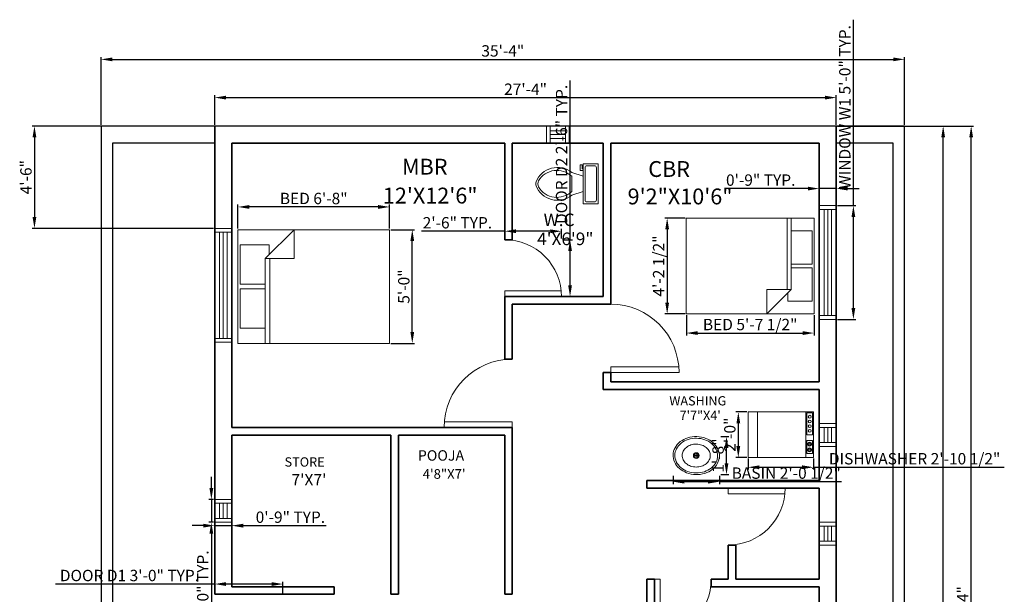
# Model space of a CAD drawing. Units: inches. Extents: x 104 to 647, y -91 to 674.
# Tile 3 of 3: x 109 to 628, y 371 to 674. Entities that reach past the tile are written whole.
import ezdxf

# ---------------------------------------------------------------- set-up
doc = ezdxf.new("R2010")
doc.units = ezdxf.units.IN
for name, color, linetype, lineweight in [('A-ANNO-DIMS', 2, 'Continuous', 18), ('A-AREA-IDEN', 7, 'Continuous', 18), ('A-DOOR', 3, 'Continuous', 18), ('A-EQPM', 8, 'Continuous', 18), ('A-FLOR-FIXT', 9, 'Continuous', 18), ('A-FURN', 8, 'Continuous', 18), ('A-GLAZ', 4, 'Continuous', 18), ('A-WALL', 7, 'Continuous', 35), ('C-PROP', 7, 'Continuous', 25)]:
    doc.layers.add(name, color=color, linetype=linetype, lineweight=lineweight)
doc.styles.get("Standard").update_dxf_attribs({"font": 'arial.ttf'})
doc.dimstyles.new('ISO-25', dxfattribs={"dimtxt": 6, "dimasz": 6, "dimexe": 1.25, "dimexo": 0.625, "dimtad": 1, "dimdec": 1, "dimlunit": 3, "dimtxsty": 'Standard', "dimcen": 2.5, "dimadec": 0, "dimazin": 0, "dimtfac": 1, "dimtdec": 1, "dimtmove": 0, "dimatfit": 3, "dimfxl": 1, "dimarcsym": 0})

# ---------------------------------------------------------------- blocks, each defined once
blk = doc.blocks.new('Bed - Queen')
for p, q in [((0, -80.00003), (0, 0)), ((0, 0), (59.99999, 0)), ((59.99999, 0), (59.99999, -80.00003)), ((7.99999, -1.2), (28.79998, -1.2)), ((7.99999, -14.4), (7.99999, -1.2)), ((28.79998, -1.2), (28.79998, -14.4)), ((31.19999, -1.2), (51.99999, -1.2)), ((31.19999, -14.4), (31.19999, -1.2)), ((51.99999, -1.2), (51.99999, -16.4)), ((0, -14.4), (44.8, -14.4)), ((59.99999, -29.6), (44.8, -14.4)), ((44.8, -14.4), (44.8, -29.6)), ((44.8, -16.8), (0, -16.8)), ((51.99999, -16.4), (46.79936, -16.4)), ((44.8, -29.6), (59.99999, -29.6)), ((59.99999, -80.00003), (0, -80.00003))]:
    blk.add_line(p, q)
blk = doc.blocks.new('Sink - Oval top')
for p, q in [((-1, 0), (1, 0)), ((0, 1), (0, -1))]:
    blk.add_line(p, q)
for points in [[(-12.23, 0.39, 0.117634), (-11.46, -3.36, 0.104469), (-8.88, -6.8, 0.090016), (-5.08, -9.07, 0.08192), (-0.32, -10.02, 0.08192), (4.49, -9.38, 0.090016), (8.42, -7.36, 0.104469), (11.22, -4.09, 0.117634), (12.23, -0.39, 0.117634), (11.46, 3.36, 0.104469), (8.88, 6.8, 0.090016), (5.08, 9.07, 0.08192), (0.32, 10.02, 0.08192), (-4.49, 9.38, 0.090016), (-8.42, 7.36, 0.104469), (-11.22, 4.09, 0.117634)], [(-11.29, 0.16, 0.118622), (-10.52, -3.25, 0.104678), (-8.07, -6.36, 0.089562), (-4.54, -8.37, 0.081185), (-0.13, -9.15, 0.081185), (4.3, -8.49, 0.089562), (7.89, -6.58, 0.104678), (10.42, -3.55, 0.118622), (11.29, -0.16, 0.118622), (10.52, 3.25, 0.104678), (8.07, 6.36, 0.089562), (4.54, 8.37, 0.081185), (0.13, 9.15, 0.081185), (-4.3, 8.49, 0.089562), (-7.89, 6.58, 0.104678), (-10.42, 3.55, 0.118622)], [(-7.42, 0.08, 0.118283), (-6.91, -2.17, 0.104607), (-5.29, -4.21, 0.089718), (-2.97, -5.53, 0.081436), (-0.07, -6.04, 0.081436), (2.84, -5.59, 0.089718), (5.2, -4.33, 0.104607), (6.86, -2.32, 0.118283), (7.42, -0.08, 0.118283), (6.91, 2.17, 0.104607), (5.29, 4.21, 0.089718), (2.97, 5.53, 0.081436), (0.07, 6.04, 0.081436), (-2.84, 5.59, 0.089718), (-5.2, 4.33, 0.104607), (-6.86, 2.32, 0.118283)]]:
    blk.add_lwpolyline(points, format="xyb", close=True)
for radius in [1.5, 1]:
    blk.add_circle((0, 0), radius)
blk = doc.blocks.new('Dishwasher')
for p, q in [((16, 32.5), (16.75, 32.5)), ((16.5, 32), (16.2942, 31.7942)), ((16.3156, 33.1843), (16.5, 33)), ((17, 32.75), (17, 33.5)), ((17, 32.25), (17, 31.5)), ((18, 32.5), (17.25, 32.5)), ((17.5, 33), (17.6938, 33.1938)), ((17.7061, 31.7939), (17.5, 32)), ((19, 32.5), (19.75, 32.5)), ((19.5, 32), (19.2942, 31.7942)), ((19.3156, 33.1843), (19.5, 33)), ((20, 32.75), (20, 33.5)), ((20, 32.25), (20, 31.5)), ((21, 32.5), (20.25, 32.5)), ((20.5, 33), (20.6938, 33.1938)), ((20.7061, 31.7939), (20.5, 32)), ((24, 30.5), (0, 30.5)), ((0, 5), (24, 5))]:
    blk.add_line(p, q)
for points in [[(0, 0), (0, 34.5), (24, 34.5), (24, 0)], [(0.5, 31), (0.5, 34), (12, 34), (12, 31)], [(15, 31), (15, 34), (22, 34), (22, 31)]]:
    blk.add_lwpolyline(points, close=True)
for centre, radius in [((2.5, 32.5), 0.75), ((5, 32.5), 0.75), ((7.5, 32.5), 0.75), ((10, 32.5), 0.75), ((17, 32.5), 1), ((20, 32.5), 1)]:
    blk.add_circle(centre, radius)
blk = doc.blocks.new('Toilet - top')
for p, q in [((9.5, -6), (9.5, -2)), ((-10, -8.5), (-8, -8.5)), ((-10, -9.5), (-10, -8.5)), ((-7, -9.5), (-10, -9.5)), ((-8, -8.5), (-8, -8)), ((-7, -8), (-7, -9.5)), ((-4, -8), (-6, -14)), ((4, -8), (6, -14)), ((4, -14), (-4, -14))]:
    blk.add_line(p, q)
blk.add_lwpolyline([(10.5, -8), (10.5, 0), (-10.5, 0), (-10.5, -8)], close=True)
for points in [[(-9.5, -2), (-9.5, -6)], [(8.5, -1), (-8.5, -1)], [(-8.5, -7), (8.5, -7)]]:
    blk.add_lwpolyline(points)
for centre, radius, start, end in [((-8.62, -1.88), 0.884, 81.8699, 188.1301), ((8.62, -1.88), 0.884, 351.8699, 98.1301), ((-8.62, -6.12), 0.884, 171.8699, 278.1301), ((8.62, -6.12), 0.884, 261.8699, 8.1301), ((3.52, -21.58), 12.17, 141.4691, 247.9714), ((4.2, -21.82), 11.33, 136.3677, 238.9468), ((-3.52, -21.58), 12.17, 292.0284, 38.5307), ((-4.2, -21.82), 11.33, 301.053, 43.6321), ((0, -27.88), 4, 245.7318, 294.2682), ((0, -29), 4, 254.8605, 285.1395)]:
    blk.add_arc(centre, radius, start, end)
blk = doc.blocks.new('*D11')
at = {"layer": 'A-ANNO-DIMS', "color": 0, "lineweight": -2, "transparency": 16777216}
for p, q in [((211.79, 618.42), (211.79, 634.03)), ((539.79, 618.42), (539.79, 634.03)), ((217.79, 632.78), (533.79, 632.78))]:
    blk.add_line(p, q, dxfattribs=at)
at = {"layer": 'A-ANNO-DIMS', "color": 0, "transparency": 16777216}
for points in [[(217.79, 633.78), (217.79, 631.78), (211.79, 632.78)], [(533.79, 633.78), (533.79, 631.78), (539.79, 632.78)]]:
    blk.add_solid(points, dxfattribs=at)
at = {"layer": 'Defpoints', "color": 0, "transparency": 16777216}
for p in [(539.79, 632.78), (211.79, 617.8), (539.79, 617.8)]:
    blk.add_point(p, dxfattribs=at)
at = {"layer": 'A-ANNO-DIMS', "color": 0, "transparency": 16777216, "insert": (375.79, 636.42), "char_height": 6, "attachment_point": 5}
blk.add_mtext('27\'-4"', dxfattribs=at)
blk = doc.blocks.new('*D12')
at = {"layer": 'A-ANNO-DIMS', "color": 0, "lineweight": -2, "transparency": 16777216}
for p, q in [((576.41, 617.8), (597.43, 617.8)), ((596.18, -48.2), (596.18, 611.8)), ((576.41, -54.2), (597.43, -54.2))]:
    blk.add_line(p, q, dxfattribs=at)
at = {"layer": 'A-ANNO-DIMS', "color": 0, "transparency": 16777216}
for points in [[(595.18, 611.8), (597.18, 611.8), (596.18, 617.8)], [(595.18, -48.2), (597.18, -48.2), (596.18, -54.2)]]:
    blk.add_solid(points, dxfattribs=at)
at = {"layer": 'Defpoints', "color": 0, "transparency": 16777216}
for p in [(575.79, 617.8), (596.18, 617.8), (575.79, -54.2)]:
    blk.add_point(p, dxfattribs=at)
at = {"layer": 'A-ANNO-DIMS', "color": 0, "transparency": 16777216, "insert": (592.49, 281.8), "char_height": 6, "attachment_point": 5, "rotation": 90}
blk.add_mtext("56'", dxfattribs=at)
blk = doc.blocks.new('WIN-60IN')
for p, q in [((60, 9), (0, 9)), ((0, 9), (0, 0)), ((2, 9), (2, 0)), ((2, 6.5), (58, 6.5)), ((58, 0), (58, 9)), ((60, 0), (60, 9)), ((0, 0), (60, 0)), ((2, 4.5), (58, 4.5)), ((2, 2.5), (58, 2.5))]:
    blk.add_line(p, q)
blk = doc.blocks.new('WIN-12IN')
for p, q in [((12, 9), (0, 9)), ((0, 9), (0, 0)), ((2, 9), (2, 0)), ((2, 6.5), (10, 6.5)), ((10, 0), (10, 9)), ((12, 0), (12, 9)), ((0, 0), (12, 0)), ((2, 4.5), (10, 4.5)), ((2, 2.5), (10, 2.5))]:
    blk.add_line(p, q)
blk = doc.blocks.new('DOOR-SWING-36IN')
for p, q in [((0, 3), (36, 3)), ((0, 0), (36, 0)), ((36, 0), (36, 3))]:
    blk.add_line(p, q)
blk.add_arc((36, 0), 36, 90, 180)
blk = doc.blocks.new('DOOR-SWING-30IN')
for p, q in [((0, 0), (0, 30)), ((0, 30), (3, 30)), ((3, 0), (3, 30))]:
    blk.add_line(p, q)
blk.add_arc((0, 30), 30, 270, 0)
blk = doc.blocks.new('*D21')
at = {"layer": 'A-ANNO-DIMS', "color": 0, "lineweight": -2, "transparency": 16777216}
for p, q in [((224.02, 563.73), (224.02, 576.36)), ((298.02, 575.11), (230.02, 575.11)), ((304.02, 563.73), (304.02, 576.36))]:
    blk.add_line(p, q, dxfattribs=at)
at = {"layer": 'A-ANNO-DIMS', "color": 0, "transparency": 16777216}
for points in [[(230.02, 576.11), (230.02, 574.11), (224.02, 575.11)], [(298.02, 576.11), (298.02, 574.11), (304.02, 575.11)]]:
    blk.add_solid(points, dxfattribs=at)
at = {"layer": 'Defpoints', "color": 0, "transparency": 16777216}
for p in [(224.02, 575.11), (224.02, 563.11), (304.02, 563.11)]:
    blk.add_point(p, dxfattribs=at)
at = {"layer": 'A-ANNO-DIMS', "color": 0, "transparency": 16777216, "insert": (264.02, 578.8), "char_height": 6, "attachment_point": 5}
blk.add_mtext('BED 6\'-8"', dxfattribs=at)
blk = doc.blocks.new('*D22')
at = {"layer": 'A-ANNO-DIMS', "color": 0, "lineweight": -2, "transparency": 16777216}
for p, q in [((304.65, 563.11), (317.27, 563.11)), ((316.02, 509.11), (316.02, 557.11)), ((304.65, 503.11), (317.27, 503.11))]:
    blk.add_line(p, q, dxfattribs=at)
at = {"layer": 'A-ANNO-DIMS', "color": 0, "transparency": 16777216}
for points in [[(315.02, 557.11), (317.02, 557.11), (316.02, 563.11)], [(315.02, 509.11), (317.02, 509.11), (316.02, 503.11)]]:
    blk.add_solid(points, dxfattribs=at)
at = {"layer": 'Defpoints', "color": 0, "transparency": 16777216}
for p in [(304.02, 563.11), (316.02, 563.11), (304.02, 503.11)]:
    blk.add_point(p, dxfattribs=at)
at = {"layer": 'A-ANNO-DIMS', "color": 0, "transparency": 16777216, "insert": (312.33, 533.11), "char_height": 6, "attachment_point": 5, "rotation": 90}
blk.add_mtext('5\'-0"', dxfattribs=at)
blk = doc.blocks.new('*D23')
at = {"layer": 'A-ANNO-DIMS', "color": 0, "lineweight": -2, "transparency": 16777216}
for p, q in [((460.64, 518.07), (460.64, 507.33)), ((528.02, 518.07), (528.02, 507.33)), ((466.64, 508.58), (522.02, 508.58))]:
    blk.add_line(p, q, dxfattribs=at)
at = {"layer": 'A-ANNO-DIMS', "color": 0, "transparency": 16777216}
for points in [[(466.64, 509.58), (466.64, 507.58), (460.64, 508.58)], [(522.02, 509.58), (522.02, 507.58), (528.02, 508.58)]]:
    blk.add_solid(points, dxfattribs=at)
at = {"layer": 'Defpoints', "color": 0, "transparency": 16777216}
for p in [(460.64, 518.69), (528.02, 518.69), (528.02, 508.58)]:
    blk.add_point(p, dxfattribs=at)
at = {"layer": 'A-ANNO-DIMS', "color": 0, "transparency": 16777216, "insert": (494.33, 512.31), "char_height": 6, "attachment_point": 5}
blk.add_mtext('BED 5\'-7 1/2"', dxfattribs=at)
blk = doc.blocks.new('*D24')
at = {"layer": 'A-ANNO-DIMS', "color": 0, "lineweight": -2, "transparency": 16777216}
for p, q in [((460.01, 569.23), (449.28, 569.23)), ((450.53, 563.23), (450.53, 524.69)), ((460.01, 518.69), (449.28, 518.69))]:
    blk.add_line(p, q, dxfattribs=at)
at = {"layer": 'A-ANNO-DIMS', "color": 0, "transparency": 16777216}
for points in [[(449.53, 563.23), (451.53, 563.23), (450.53, 569.23)], [(449.53, 524.69), (451.53, 524.69), (450.53, 518.69)]]:
    blk.add_solid(points, dxfattribs=at)
at = {"layer": 'Defpoints', "color": 0, "transparency": 16777216}
for p in [(460.64, 569.23), (450.53, 518.69), (460.64, 518.69)]:
    blk.add_point(p, dxfattribs=at)
at = {"layer": 'A-ANNO-DIMS', "color": 0, "transparency": 16777216, "insert": (446.8, 543.96), "char_height": 6, "attachment_point": 5, "rotation": 90}
blk.add_mtext('4\'-2 1/2"', dxfattribs=at)
blk = doc.blocks.new('*D27')
at = {"layer": 'A-ANNO-DIMS', "color": 0, "lineweight": -2, "transparency": 16777216}
for p, q in [((548.79, 575.8), (548.79, 673.87)), ((540.41, 575.8), (550.04, 575.8)), ((548.79, 521.8), (548.79, 569.8)), ((540.41, 515.8), (550.04, 515.8))]:
    blk.add_line(p, q, dxfattribs=at)
at = {"layer": 'A-ANNO-DIMS', "color": 0, "transparency": 16777216}
for points in [[(547.79, 569.8), (549.79, 569.8), (548.79, 575.8)], [(547.79, 521.8), (549.79, 521.8), (548.79, 515.8)]]:
    blk.add_solid(points, dxfattribs=at)
at = {"layer": 'Defpoints', "color": 0, "transparency": 16777216}
for p in [(539.79, 575.8), (548.79, 575.8), (539.79, 515.8)]:
    blk.add_point(p, dxfattribs=at)
at = {"layer": 'A-ANNO-DIMS', "color": 0, "transparency": 16777216, "insert": (545.06, 627.84), "char_height": 6, "attachment_point": 5, "rotation": 90}
blk.add_mtext('WINDOW W1 5\'-0" TYP.', dxfattribs=at)
blk = doc.blocks.new('*D28')
at = {"layer": 'A-ANNO-DIMS', "color": 0, "lineweight": -2, "transparency": 16777216}
for p, q in [((524.79, 584.8), (480.97, 584.8)), ((530.79, 576.42), (530.79, 586.05)), ((539.79, 584.8), (530.79, 584.8)), ((539.79, 576.42), (539.79, 586.05)), ((545.79, 584.8), (551.79, 584.8))]:
    blk.add_line(p, q, dxfattribs=at)
at = {"layer": 'A-ANNO-DIMS', "color": 0, "transparency": 16777216}
for points in [[(524.79, 585.8), (524.79, 583.8), (530.79, 584.8)], [(545.79, 585.8), (545.79, 583.8), (539.79, 584.8)]]:
    blk.add_solid(points, dxfattribs=at)
at = {"layer": 'Defpoints', "color": 0, "transparency": 16777216}
for p in [(530.79, 584.8), (530.79, 575.8), (539.79, 575.8)]:
    blk.add_point(p, dxfattribs=at)
at = {"layer": 'A-ANNO-DIMS', "color": 0, "transparency": 16777216, "insert": (499.88, 588.49), "char_height": 6, "attachment_point": 5}
blk.add_mtext('0\'-9" TYP.', dxfattribs=at)
blk = doc.blocks.new('*D29')
at = {"layer": 'A-ANNO-DIMS', "color": 0, "lineweight": -2, "transparency": 16777216}
for p, q in [((209.99, 426.8), (209.99, 432.8)), ((211.16, 420.8), (208.74, 420.8)), ((209.99, 420.8), (209.99, 408.8)), ((211.16, 408.8), (208.74, 408.8)), ((209.99, 402.8), (209.99, 304.72))]:
    blk.add_line(p, q, dxfattribs=at)
at = {"layer": 'A-ANNO-DIMS', "color": 0, "transparency": 16777216}
for points in [[(208.99, 426.8), (210.99, 426.8), (209.99, 420.8)], [(208.99, 402.8), (210.99, 402.8), (209.99, 408.8)]]:
    blk.add_solid(points, dxfattribs=at)
at = {"layer": 'Defpoints', "color": 0, "transparency": 16777216}
for p in [(211.79, 420.8), (209.99, 408.8), (211.79, 408.8)]:
    blk.add_point(p, dxfattribs=at)
at = {"layer": 'A-ANNO-DIMS', "color": 0, "transparency": 16777216, "insert": (206.26, 350.76), "char_height": 6, "attachment_point": 5, "rotation": 90}
blk.add_mtext('WINDOW W2 1\'-0" TYP.', dxfattribs=at)
blk = doc.blocks.new('*D30')
at = {"layer": 'A-ANNO-DIMS', "color": 0, "lineweight": -2, "transparency": 16777216}
for p, q in [((205.79, 407), (199.79, 407)), ((211.79, 408.17), (211.79, 405.75)), ((211.79, 407), (220.79, 407)), ((220.79, 408.17), (220.79, 405.75)), ((226.79, 407), (270.61, 407))]:
    blk.add_line(p, q, dxfattribs=at)
at = {"layer": 'A-ANNO-DIMS', "color": 0, "transparency": 16777216}
for points in [[(205.79, 408), (205.79, 406), (211.79, 407)], [(226.79, 408), (226.79, 406), (220.79, 407)]]:
    blk.add_solid(points, dxfattribs=at)
at = {"layer": 'Defpoints', "color": 0, "transparency": 16777216}
for p in [(211.79, 408.8), (220.79, 408.8), (220.79, 407)]:
    blk.add_point(p, dxfattribs=at)
at = {"layer": 'A-ANNO-DIMS', "color": 0, "transparency": 16777216, "insert": (251.7, 410.69), "char_height": 6, "attachment_point": 5}
blk.add_mtext('0\'-9" TYP.', dxfattribs=at)
blk = doc.blocks.new('*D31')
at = {"layer": 'A-ANNO-DIMS', "color": 0, "lineweight": -2, "transparency": 16777216}
for p, q in [((211.79, 376.2), (127.75, 376.2)), ((211.79, 371.42), (211.79, 377.45)), ((241.79, 376.2), (217.79, 376.2)), ((247.79, 371.42), (247.79, 377.45))]:
    blk.add_line(p, q, dxfattribs=at)
at = {"layer": 'A-ANNO-DIMS', "color": 0, "transparency": 16777216}
for points in [[(217.79, 377.2), (217.79, 375.2), (211.79, 376.2)], [(241.79, 377.2), (241.79, 375.2), (247.79, 376.2)]]:
    blk.add_solid(points, dxfattribs=at)
at = {"layer": 'Defpoints', "color": 0, "transparency": 16777216}
for p in [(211.79, 376.2), (211.79, 370.8), (247.79, 370.8)]:
    blk.add_point(p, dxfattribs=at)
at = {"layer": 'A-ANNO-DIMS', "color": 0, "transparency": 16777216, "insert": (166.77, 379.93), "char_height": 6, "attachment_point": 5}
blk.add_mtext('DOOR D1 3\'-0" TYP.', dxfattribs=at)
blk = doc.blocks.new('*D33')
at = {"layer": 'A-ANNO-DIMS', "color": 0, "lineweight": -2, "transparency": 16777216}
for p, q in [((399.29, 557.8), (399.29, 641.84)), ((395.41, 557.8), (400.54, 557.8)), ((399.29, 533.8), (399.29, 551.8)), ((395.41, 527.8), (400.54, 527.8))]:
    blk.add_line(p, q, dxfattribs=at)
at = {"layer": 'A-ANNO-DIMS', "color": 0, "transparency": 16777216}
for points in [[(398.29, 551.8), (400.29, 551.8), (399.29, 557.8)], [(398.29, 533.8), (400.29, 533.8), (399.29, 527.8)]]:
    blk.add_solid(points, dxfattribs=at)
at = {"layer": 'Defpoints', "color": 0, "transparency": 16777216}
for p in [(394.79, 557.8), (399.29, 557.8), (394.79, 527.8)]:
    blk.add_point(p, dxfattribs=at)
at = {"layer": 'A-ANNO-DIMS', "color": 0, "transparency": 16777216, "insert": (395.56, 602.82), "char_height": 6, "attachment_point": 5, "rotation": 90}
blk.add_mtext('DOOR D2 2\'-6" TYP.', dxfattribs=at)
blk = doc.blocks.new('*D34')
at = {"layer": 'A-ANNO-DIMS', "color": 0, "lineweight": -2, "transparency": 16777216}
for p, q in [((364.79, 562.3), (320.86, 562.3)), ((364.79, 558.42), (364.79, 563.55)), ((388.79, 562.3), (370.79, 562.3)), ((394.79, 558.42), (394.79, 563.55))]:
    blk.add_line(p, q, dxfattribs=at)
at = {"layer": 'A-ANNO-DIMS', "color": 0, "transparency": 16777216}
for points in [[(370.79, 563.3), (370.79, 561.3), (364.79, 562.3)], [(388.79, 563.3), (388.79, 561.3), (394.79, 562.3)]]:
    blk.add_solid(points, dxfattribs=at)
at = {"layer": 'Defpoints', "color": 0, "transparency": 16777216}
for p in [(364.79, 562.3), (364.79, 557.8), (394.79, 557.8)]:
    blk.add_point(p, dxfattribs=at)
at = {"layer": 'A-ANNO-DIMS', "color": 0, "transparency": 16777216, "insert": (339.83, 565.99), "char_height": 6, "attachment_point": 5}
blk.add_mtext('2\'-6" TYP.', dxfattribs=at)
blk = doc.blocks.new('*D41')
at = {"layer": 'A-ANNO-DIMS', "color": 0, "lineweight": -2, "transparency": 16777216}
for p, q in [((453.61, 433.28), (453.61, 428.97)), ((478.16, 433.28), (478.16, 428.97)), ((459.61, 430.22), (472.16, 430.22)), ((478.16, 430.22), (542.56, 430.22))]:
    blk.add_line(p, q, dxfattribs=at)
at = {"layer": 'A-ANNO-DIMS', "color": 0, "transparency": 16777216}
for points in [[(459.61, 431.22), (459.61, 429.22), (453.61, 430.22)], [(472.16, 431.22), (472.16, 429.22), (478.16, 430.22)]]:
    blk.add_solid(points, dxfattribs=at)
at = {"layer": 'Defpoints', "color": 0, "transparency": 16777216}
for p in [(453.61, 433.9), (478.16, 433.9), (478.16, 430.22)]:
    blk.add_point(p, dxfattribs=at)
at = {"layer": 'A-ANNO-DIMS', "color": 0, "transparency": 16777216, "insert": (513.36, 433.94), "char_height": 6, "attachment_point": 5}
blk.add_mtext('BASIN 2\'-0 1/2"', dxfattribs=at)
blk = doc.blocks.new('*D42')
at = {"layer": 'A-ANNO-DIMS', "color": 0, "lineweight": -2, "transparency": 16777216}
for p, q in [((478.78, 454.04), (483.09, 454.04)), ((481.84, 439.9), (481.84, 448.04)), ((478.78, 433.9), (483.09, 433.9))]:
    blk.add_line(p, q, dxfattribs=at)
at = {"layer": 'A-ANNO-DIMS', "color": 0, "transparency": 16777216}
for points in [[(480.84, 448.04), (482.84, 448.04), (481.84, 454.04)], [(480.84, 439.9), (482.84, 439.9), (481.84, 433.9)]]:
    blk.add_solid(points, dxfattribs=at)
at = {"layer": 'Defpoints', "color": 0, "transparency": 16777216}
for p in [(478.16, 454.04), (481.84, 454.04), (478.16, 433.9)]:
    blk.add_point(p, dxfattribs=at)
at = {"layer": 'A-ANNO-DIMS', "color": 0, "transparency": 16777216, "insert": (478.15, 443.97), "char_height": 6, "attachment_point": 5, "rotation": 90}
blk.add_mtext('1\'-8"', dxfattribs=at)
blk = doc.blocks.new('*D47')
at = {"layer": 'A-ANNO-DIMS', "color": 0, "lineweight": -2, "transparency": 16777216}
for p, q in [((493.24, 442.35), (493.24, 436.55)), ((527.74, 442.35), (527.74, 436.55)), ((499.24, 437.8), (521.74, 437.8)), ((527.74, 437.8), (628.43, 437.8))]:
    blk.add_line(p, q, dxfattribs=at)
at = {"layer": 'A-ANNO-DIMS', "color": 0, "transparency": 16777216}
for points in [[(499.24, 438.8), (499.24, 436.8), (493.24, 437.8)], [(521.74, 438.8), (521.74, 436.8), (527.74, 437.8)]]:
    blk.add_solid(points, dxfattribs=at)
at = {"layer": 'Defpoints', "color": 0, "transparency": 16777216}
for p in [(493.24, 442.98), (527.74, 442.98), (527.74, 437.8)]:
    blk.add_point(p, dxfattribs=at)
at = {"layer": 'A-ANNO-DIMS', "color": 0, "transparency": 16777216, "insert": (581.09, 441.53), "char_height": 6, "attachment_point": 5}
blk.add_mtext('DISHWASHER 2\'-10 1/2"', dxfattribs=at)
blk = doc.blocks.new('*D48')
at = {"layer": 'A-ANNO-DIMS', "color": 0, "lineweight": -2, "transparency": 16777216}
for p, q in [((492.62, 466.98), (486.82, 466.98)), ((488.07, 460.98), (488.07, 448.98)), ((492.62, 442.98), (486.82, 442.98))]:
    blk.add_line(p, q, dxfattribs=at)
at = {"layer": 'A-ANNO-DIMS', "color": 0, "transparency": 16777216}
for points in [[(487.07, 460.98), (489.07, 460.98), (488.07, 466.98)], [(487.07, 448.98), (489.07, 448.98), (488.07, 442.98)]]:
    blk.add_solid(points, dxfattribs=at)
at = {"layer": 'Defpoints', "color": 0, "transparency": 16777216}
for p in [(493.24, 466.98), (488.07, 442.98), (493.24, 442.98)]:
    blk.add_point(p, dxfattribs=at)
at = {"layer": 'A-ANNO-DIMS', "color": 0, "transparency": 16777216, "insert": (484.38, 454.98), "char_height": 6, "attachment_point": 5, "rotation": 90}
blk.add_mtext('2\'-0"', dxfattribs=at)
blk = doc.blocks.new('*D51')
at = {"layer": 'A-ANNO-DIMS', "color": 0, "lineweight": -2, "transparency": 16777216}
for p, q in [((151.79, 618.42), (151.79, 654.2)), ((157.79, 652.95), (569.79, 652.95)), ((575.79, 618.42), (575.79, 654.2))]:
    blk.add_line(p, q, dxfattribs=at)
at = {"layer": 'A-ANNO-DIMS', "color": 0, "transparency": 16777216}
for points in [[(157.79, 653.95), (157.79, 651.95), (151.79, 652.95)], [(569.79, 653.95), (569.79, 651.95), (575.79, 652.95)]]:
    blk.add_solid(points, dxfattribs=at)
at = {"layer": 'Defpoints', "color": 0, "transparency": 16777216}
for p in [(575.79, 652.95), (151.79, 617.8), (575.79, 617.8)]:
    blk.add_point(p, dxfattribs=at)
at = {"layer": 'A-ANNO-DIMS', "color": 0, "transparency": 16777216, "insert": (363.79, 656.64), "char_height": 6, "attachment_point": 5}
blk.add_mtext('35\'-4"', dxfattribs=at)
blk = doc.blocks.new('*D52')
at = {"layer": 'A-ANNO-DIMS', "color": 0, "lineweight": -2, "transparency": 16777216}
for p, q in [((540.41, 617.8), (612.19, 617.8)), ((610.94, 115.8), (610.94, 611.8)), ((540.41, 109.8), (612.19, 109.8))]:
    blk.add_line(p, q, dxfattribs=at)
at = {"layer": 'A-ANNO-DIMS', "color": 0, "transparency": 16777216}
for points in [[(609.94, 611.8), (611.94, 611.8), (610.94, 617.8)], [(609.94, 115.8), (611.94, 115.8), (610.94, 109.8)]]:
    blk.add_solid(points, dxfattribs=at)
at = {"layer": 'Defpoints', "color": 0, "transparency": 16777216}
for p in [(539.79, 617.8), (610.94, 617.8), (539.79, 109.8)]:
    blk.add_point(p, dxfattribs=at)
at = {"layer": 'A-ANNO-DIMS', "color": 0, "transparency": 16777216, "insert": (607.3, 363.8), "char_height": 6, "attachment_point": 5, "rotation": 90}
blk.add_mtext('42\'-4"', dxfattribs=at)
blk = doc.blocks.new('*D57')
at = {"layer": 'A-ANNO-DIMS', "color": 0, "lineweight": -2, "transparency": 16777216}
for p, q in [((211.16, 617.8), (115.39, 617.8)), ((116.64, 611.8), (116.64, 569.8)), ((211.16, 563.8), (115.39, 563.8))]:
    blk.add_line(p, q, dxfattribs=at)
at = {"layer": 'A-ANNO-DIMS', "color": 0, "transparency": 16777216}
for points in [[(115.64, 611.8), (117.64, 611.8), (116.64, 617.8)], [(115.64, 569.8), (117.64, 569.8), (116.64, 563.8)]]:
    blk.add_solid(points, dxfattribs=at)
at = {"layer": 'Defpoints', "color": 0, "transparency": 16777216}
for p in [(211.79, 617.8), (116.64, 563.8), (211.79, 563.8)]:
    blk.add_point(p, dxfattribs=at)
at = {"layer": 'A-ANNO-DIMS', "color": 0, "transparency": 16777216, "insert": (112.95, 590.8), "char_height": 6, "attachment_point": 5, "rotation": 90}
blk.add_mtext('4\'-6"', dxfattribs=at)

msp = doc.modelspace()

# ---------------------------------------------------------------- linework, layer by layer
at = {"layer": 'A-WALL'}
for p, q in [((211.79, 608.8), (211.79, 617.8)), ((539.79, 608.8), (539.79, 617.8)), ((211.79, 608.8), (211.79, 370.8)), ((220.79, 608.8), (220.79, 458.8)), ((364.79, 608.8), (220.79, 608.8)), ((364.79, 608.8), (364.79, 557.8)), ((364.79, 608.8), (364.79, 557.8)), ((368.79, 608.8), (368.79, 557.8)), ((368.79, 608.8), (368.79, 557.8)), ((416.79, 608.8), (368.79, 608.8)), ((416.79, 608.8), (416.79, 527.8)), ((420.79, 608.8), (420.79, 523.8)), ((530.79, 608.8), (420.79, 608.8)), ((530.79, 482.8), (530.79, 608.8)), ((539.79, 109.8), (539.79, 608.8)), ((368.79, 557.8), (364.79, 557.8)), ((416.79, 527.8), (364.79, 527.8)), ((364.79, 527.8), (364.79, 494.8)), ((364.79, 527.8), (364.79, 494.8)), ((420.79, 523.8), (368.79, 523.8)), ((368.79, 523.8), (368.79, 494.8)), ((368.79, 523.8), (368.79, 494.8)), ((368.79, 494.8), (364.79, 494.8)), ((416.79, 487.8), (416.79, 478.8)), ((420.79, 487.8), (416.79, 487.8)), ((420.79, 487.8), (420.79, 482.8)), ((530.79, 478.8), (416.79, 478.8)), ((530.79, 482.8), (420.79, 482.8)), ((530.79, 430.8), (530.79, 478.8)), ((368.79, 458.8), (220.79, 458.8)), ((368.79, 458.8), (368.79, 370.8)), ((368.79, 458.8), (368.79, 370.8)), ((220.79, 454.8), (220.79, 374.8)), ((304.79, 454.8), (220.79, 454.8)), ((304.79, 454.8), (304.79, 370.8)), ((364.79, 454.8), (308.79, 454.8)), ((308.79, 454.8), (308.79, 370.8)), ((364.79, 454.8), (364.79, 370.8)), ((364.79, 454.8), (364.79, 370.8)), ((530.79, 430.8), (439.79, 430.8)), ((439.79, 426.8), (439.79, 430.8)), ((530.79, 426.8), (439.79, 426.8)), ((530.79, 378.8), (530.79, 426.8)), ((486.79, 396.8), (482.79, 396.8)), ((482.79, 378.8), (482.79, 396.8)), ((486.79, 378.8), (486.79, 396.8)), ((274.79, 374.8), (220.79, 374.8)), ((274.79, 374.8), (274.79, 370.8)), ((443.79, 378.8), (439.79, 378.8)), ((439.79, 326.8), (439.79, 378.8)), ((443.79, 326.8), (443.79, 378.8)), ((473.79, 374.8), (473.79, 378.8)), ((482.79, 378.8), (473.79, 378.8)), ((530.79, 374.8), (473.79, 374.8)), ((530.79, 378.8), (486.79, 378.8)), ((530.79, 326.8), (530.79, 374.8)), ((274.79, 370.8), (211.79, 370.8)), ((308.79, 370.8), (304.79, 370.8)), ((368.79, 370.8), (364.79, 370.8))]:
    msp.add_line(p, q, dxfattribs=at)
at = {"layer": 'C-PROP'}
for p, q in [((151.79, 617.8), (151.79, -54.2)), ((575.79, 617.8), (151.79, 617.8)), ((575.79, -54.2), (575.79, 617.8)), ((157.79, 608.8), (157.79, -48.2)), ((211.79, 608.8), (157.79, 608.8)), ((569.79, 608.8), (539.79, 608.8)), ((569.79, -48.2), (569.79, 608.8))]:
    msp.add_line(p, q, dxfattribs=at)

# ---------------------------------------------------------------- block references
at = {"layer": 'A-DOOR', "rotation": 90.00000000000006}
msp.add_blockref('DOOR-SWING-30IN', (394.79, 527.8), dxfattribs=at)
at = {"layer": 'A-DOOR', "extrusion": (0, 0, -1), "zscale": -1}
msp.add_blockref('DOOR-SWING-36IN', (-456.79, 487.8), dxfattribs=at)
at = {"layer": 'A-DOOR'}
for name, p in [('DOOR-SWING-36IN', (332.79, 458.8)), ('DOOR-SWING-30IN', (443.79, 348.8))]:
    msp.add_blockref(name, p, dxfattribs=at)
at = {"layer": 'A-DOOR', "extrusion": (0, 0, -1), "zscale": -1, "rotation": 270.0000000000002}
msp.add_blockref('DOOR-SWING-30IN', (-512.79, 426.8), dxfattribs=at)
at = {"layer": 'A-EQPM', "rotation": 270}
msp.add_blockref('Dishwasher', (493.24, 466.98), dxfattribs=at)
at = {"layer": 'A-FLOR-FIXT', "rotation": 270}
msp.add_blockref('Toilet - top', (414.18, 587.29), dxfattribs=at)
at = {"layer": 'A-FLOR-FIXT'}
msp.add_blockref('Sink - Oval top', (465.88, 443.97), dxfattribs=at)
at = {"layer": 'A-FURN', "xscale": 0.8423033598748597, "yscale": 0.8423033598748597, "zscale": 0.8423033598748597, "rotation": 270}
msp.add_blockref('Bed - Queen', (528.02, 569.23), dxfattribs=at)
at = {"layer": 'A-FURN', "rotation": 90}
msp.add_blockref('Bed - Queen', (224.02, 503.11), dxfattribs=at)
at = {"layer": 'A-GLAZ'}
for name, p, rotation in [('WIN-12IN', (398.79, 617.8), 180), ('WIN-60IN', (539.79, 515.8), 90.00000000000006), ('WIN-60IN', (220.79, 503.8), 90.00000000000003), ('WIN-12IN', (530.79, 460.8), 269.9999999999999), ('WIN-12IN', (211.79, 420.8), 269.9999999999994), ('WIN-12IN', (530.79, 408.8), 269.9999999999999)]:
    msp.add_blockref(name, p, dxfattribs=dict(at, rotation=rotation))

# ---------------------------------------------------------------- texts
at = {"layer": 'A-AREA-IDEN', "attachment_point": 1}
for s, width, gutter_width, insert, char_height in [('MBR', 225.5639, 41.81, (310.61, 600.53), 8.362), ('CBR', 225.5639, 41.81, (440.53, 599.3), 8.362), ('12\'X12\'6"', 225.5639, 41.81, (300.51, 585.28), 8.362), ('9\'2"X10\'6"', 225.5639, 41.81, (429.65, 584.83), 8.362), ('W.C', 179.8701, 33.34, (385.33, 571.65), 6.668), ('4\'X6\'9"', 179.8701, 33.34, (381.92, 561.63), 6.668), ('WASHING', 131.4694, 24.37, (451.67, 475.29), 4.874), ('7\'7"X4\'', 131.4694, 24.37, (457.08, 467.57), 4.874), ('POOJA', 148.3298, 27.5, (318.95, 446.78), 5.499), ('STORE', 132.3228, 24.53, (248.64, 443.05), 4.906), ('4\'8"X7\'', 136.8683, 25.37, (321.52, 436.8), 5.074), ("7'X7'", 163.1522, 30.24, (252.25, 434.24), 6.049)]:
    msp.add_mtext_dynamic_manual_height_columns(s, width=width, gutter_width=gutter_width, heights=[0], dxfattribs=dict(at, insert=insert, char_height=char_height))

# ---------------------------------------------------------------- dimensions: what is measured, and where the dimension line sits
at = {"layer": 'A-ANNO-DIMS'}
for base, p1, p2, angle, text, picture, middle in [((548.79, 575.8), (539.79, 515.8), (539.79, 575.8), 90, 'WINDOW W1 <> TYP.', '*D27', (545.06, 627.84)), ((399.29, 557.8), (394.79, 527.8), (394.79, 557.8), 90, 'DOOR D2 <> TYP.', '*D33', (395.56, 602.82)), ((530.79, 584.8), (539.79, 575.8), (530.79, 575.8), 180, '<> TYP.', '*D28', (499.88, 588.49)), ((224.02, 575.11), (304.02, 563.11), (224.02, 563.11), 180, 'BED <>', '*D21', (264.02, 578.8)), ((364.79, 562.3), (394.79, 557.8), (364.79, 557.8), 180, '<> TYP.', '*D34', (339.83, 565.99)), ((209.99, 408.8), (211.79, 420.8), (211.79, 408.8), 270, 'WINDOW W2 <> TYP.', '*D29', (206.26, 350.76)), ((211.79, 376.2), (247.79, 370.8), (211.79, 370.8), 180, 'DOOR D1 <> TYP.', '*D31', (166.77, 379.93))]:
    dim = msp.add_linear_dim(base=base, p1=p1, p2=p2, angle=angle, text=text, dimstyle='ISO-25', override={"dimdec": 1, "dimlfac": 1, "dimrnd": 0, "dimzin": 1, "dimdsep": 46, "dimlunit": 4, "dimfrac": 2}, dxfattribs=at)
    dim.commit()
    dim.dimension.update_dxf_attribs({"geometry": picture, "text_midpoint": middle})
for base, p1, p2, override, picture, middle in [((575.79, 652.95), (151.79, 617.8), (575.79, 617.8), {"dimdec": 1, "dimlfac": 1, "dimrnd": 0, "dimzin": 1, "dimdsep": 46, "dimlunit": 4, "dimfrac": 2}, '*D51', (363.79, 656.64)), ((539.79, 632.78), (211.79, 617.8), (539.79, 617.8), {"dimclrd": 0, "dimclre": 0, "dimclrt": 0}, '*D11', (375.79, 636.42))]:
    dim = msp.add_linear_dim(base=base, p1=p1, p2=p2, dimstyle='ISO-25', override=override, dxfattribs=at)
    dim.commit()
    dim.dimension.update_dxf_attribs({"geometry": picture, "text_midpoint": middle})
for base, p1, p2, angle, picture, middle in [((116.64, 563.8), (211.79, 617.8), (211.79, 563.8), 90, '*D57', (112.95, 590.8)), ((610.94, 617.8), (539.79, 109.8), (539.79, 617.8), 90, '*D52', (607.3, 363.8)), ((450.53, 518.69), (460.64, 569.23), (460.64, 518.69), 270, '*D24', (446.8, 543.96)), ((316.02, 563.11), (304.02, 503.11), (304.02, 563.11), 90, '*D22', (312.33, 533.11)), ((488.07, 442.98), (493.24, 466.98), (493.24, 442.98), 270, '*D48', (484.38, 454.98)), ((481.84, 454.04), (478.16, 433.9), (478.16, 454.04), 90, '*D42', (478.15, 443.97))]:
    dim = msp.add_linear_dim(base=base, p1=p1, p2=p2, angle=angle, dimstyle='ISO-25', override={"dimdec": 1, "dimlfac": 1, "dimrnd": 0, "dimzin": 1, "dimdsep": 46, "dimlunit": 4, "dimfrac": 2}, dxfattribs=at)
    dim.commit()
    dim.dimension.update_dxf_attribs({"geometry": picture, "text_midpoint": middle})
dim = msp.add_aligned_dim(p1=(575.79, -54.2), p2=(575.79, 617.8), distance=-20.39, dimstyle='ISO-25', override={"dimclrd": 0, "dimclre": 0, "dimclrt": 0}, dxfattribs=at)
dim.commit()
dim.dimension.update_dxf_attribs({"geometry": '*D12', "text_midpoint": (592.49, 281.8)})
for base, p1, p2, text, picture, middle in [((528.02, 508.58), (460.64, 518.69), (528.02, 518.69), 'BED <>', '*D23', (494.33, 512.31)), ((527.74, 437.8), (493.24, 442.98), (527.74, 442.98), 'DISHWASHER <>', '*D47', (581.09, 441.53)), ((478.1597, 430.2175), (453.6088, 433.9001), (478.1597, 433.9001), 'BASIN <>', '*D41', (513.3584, 433.9448)), ((220.79, 407), (211.79, 408.8), (220.79, 408.8), '<> TYP.', '*D30', (251.7, 410.69))]:
    dim = msp.add_linear_dim(base=base, p1=p1, p2=p2, text=text, dimstyle='ISO-25', override={"dimdec": 1, "dimlfac": 1, "dimrnd": 0, "dimzin": 1, "dimdsep": 46, "dimlunit": 4, "dimfrac": 2}, dxfattribs=at)
    dim.commit()
    dim.dimension.update_dxf_attribs({"geometry": picture, "text_midpoint": middle})

doc.saveas('drawing.dxf')
